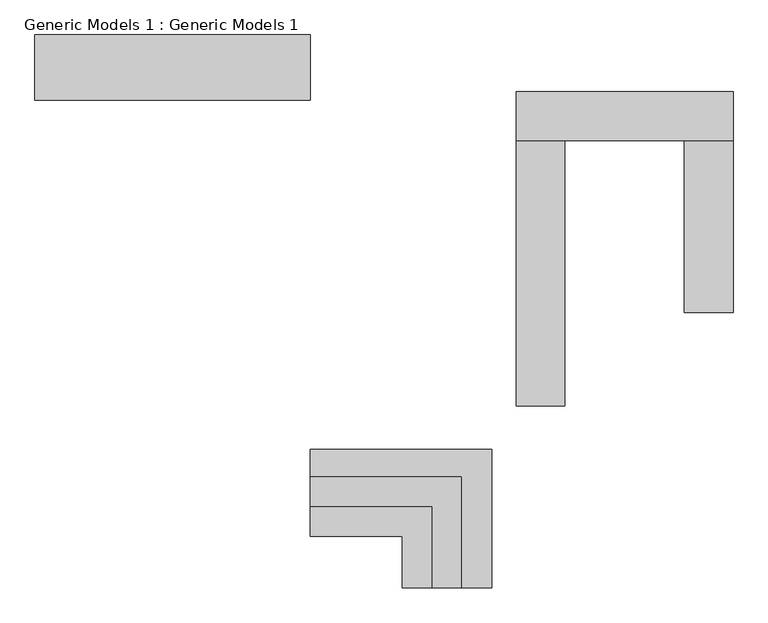
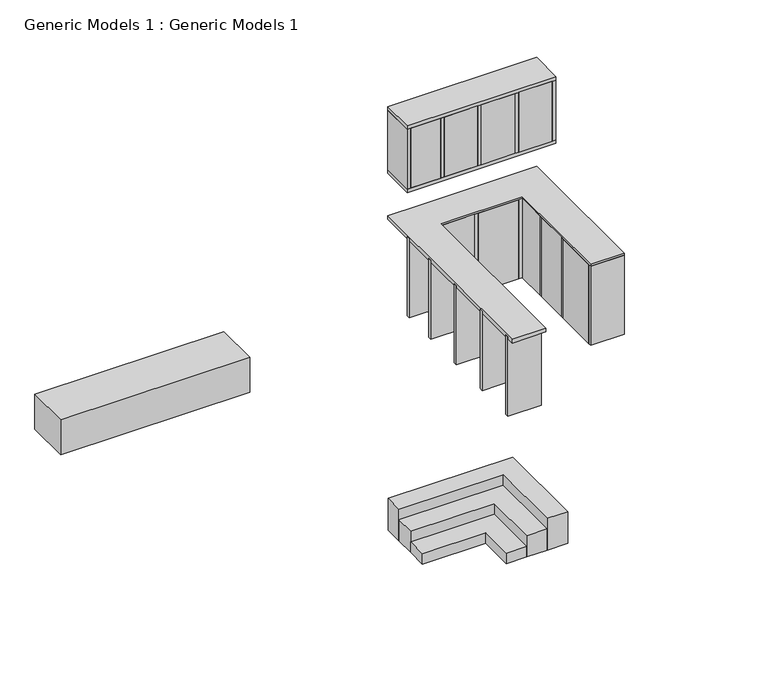
"""IFC4 building model written with IfcOpenShell, lengths in millimetres: proxy geometry, Generic Models 1 : Generic Models 1."""

from ifc_helpers import new_model, si_unit, frame, origin, place, context, project, spatial, polyline, outline, extrude, source, transform, mapped, element, save


def generic_models_1_generic_models_1_30c65cec(model_context):
    return source(origin(), model_context, "Body", "SweptSolid", [
        extrude(outline(polyline([(-6395.1591227, 5407.3642852), (-6395.1591227, 4797.7642852), (-8973.2591227, 4797.7642852), (-8973.2591227, 5407.3642852), (-6395.1591227, 5407.3642852)])), frame((0.0, 0.0, -609.6), z_axis=(0.0, 0.0, 1.0), x_axis=(1.0, 0.0, 0.0)), (0.0, 0.0, 1.0), 508.0),
        extrude(outline(polyline([(-5252.1591227, 987.7642852), (-5252.1591227, 225.7642852), (-5531.5591227, 225.7642852), (-5531.5591227, 708.3642852), (-6395.1591227, 708.3642852), (-6395.1591227, 987.7642852), (-5252.1591227, 987.7642852)])), frame((0.0, 0.0, -609.6), z_axis=(0.0, 0.0, 1.0), x_axis=(1.0, 0.0, 0.0)), (0.0, 0.0, 1.0), 152.4),
        extrude(outline(polyline([(-6395.1591227, 987.7642852), (-6395.1591227, 1267.1642852), (-4972.7591227, 1267.1642852), (-4972.7591227, 225.7642852), (-5252.1591227, 225.7642852), (-5252.1591227, 987.7642852), (-6395.1591227, 987.7642852)])), frame((0.0, 0.0, -609.6), z_axis=(0.0, 0.0, 1.0), x_axis=(1.0, 0.0, 0.0)), (0.0, 0.0, 1.0), 304.8),
        extrude(outline(polyline([(-4693.3591227, 1521.1642852), (-4693.3591227, 225.7642852), (-4972.7591227, 225.7642852), (-4972.7591227, 1267.1642852), (-6395.1591227, 1267.1642852), (-6395.1591227, 1521.1642852), (-4693.3591227, 1521.1642852)])), frame((0.0, 0.0, -609.6), z_axis=(0.0, 0.0, 1.0), x_axis=(1.0, 0.0, 0.0)), (0.0, 0.0, 1.0), 457.2),
        extrude(outline(polyline([(-4007.5591227, 4416.7642852), (-4413.9591227, 4416.7642852), (-4413.9591227, 4436.1688715), (-4007.5591227, 4436.1688715), (-4007.5591227, 4416.7642852)])), frame((0.0, 0.0, 1879.6), z_axis=(0.0, 0.0, 1.0), x_axis=(1.0, 0.0, 0.0)), (0.0, 0.0, 1.0), 863.6),
        extrude(outline(polyline([(-3499.5591227, 4416.7642852), (-3956.7591227, 4416.7642852), (-3956.7591227, 4436.1688715), (-3499.5591227, 4436.1688715), (-3499.5591227, 4416.7642852)])), frame((0.0, 0.0, 1879.6), z_axis=(0.0, 0.0, 1.0), x_axis=(1.0, 0.0, 0.0)), (0.0, 0.0, 1.0), 863.6),
        extrude(outline(polyline([(-2991.5591227, 4416.7642852), (-3448.7591227, 4416.7642852), (-3448.7591227, 4436.1688715), (-2991.5591227, 4436.1688715), (-2991.5591227, 4416.7642852)])), frame((0.0, 0.0, 1879.6), z_axis=(0.0, 0.0, 1.0), x_axis=(1.0, 0.0, 0.0)), (0.0, 0.0, 1.0), 863.6),
        extrude(outline(polyline([(-2483.5591227, 4416.7642852), (-2940.7591227, 4416.7642852), (-2940.7591227, 4436.1688715), (-2483.5591227, 4436.1688715), (-2483.5591227, 4416.7642852)])), frame((0.0, 0.0, 1879.6), z_axis=(0.0, 0.0, 1.0), x_axis=(1.0, 0.0, 0.0)), (0.0, 0.0, 1.0), 863.6),
        extrude(outline(polyline([(-2432.7591227, 4873.9642852), (-2432.7591227, 4416.7642852), (-4464.7591227, 4416.7642852), (-4464.7591227, 4873.9642852), (-2432.7591227, 4873.9642852)])), frame((0.0, 0.0, 2743.2), z_axis=(0.0, 0.0, 1.0), x_axis=(1.0, 0.0, 0.0)), (0.0, 0.0, 1.0), 50.8),
        extrude(outline(polyline([(-4413.9591227, 4873.9642852), (-4413.9591227, 4416.7642852), (-4464.7591227, 4416.7642852), (-4464.7591227, 4873.9642852), (-4413.9591227, 4873.9642852)])), frame((0.0, 0.0, 1879.6), z_axis=(0.0, 0.0, 1.0), x_axis=(1.0, 0.0, 0.0)), (0.0, 0.0, 1.0), 863.6),
        extrude(outline(polyline([(-3956.7591227, 4873.9642852), (-3956.7591227, 4416.7642852), (-4007.5591227, 4416.7642852), (-4007.5591227, 4873.9642852), (-3956.7591227, 4873.9642852)])), frame((0.0, 0.0, 1879.6), z_axis=(0.0, 0.0, 1.0), x_axis=(1.0, 0.0, 0.0)), (0.0, 0.0, 1.0), 863.6),
        extrude(outline(polyline([(-3448.7591227, 4873.9642852), (-3448.7591227, 4416.7642852), (-3499.5591227, 4416.7642852), (-3499.5591227, 4873.9642852), (-3448.7591227, 4873.9642852)])), frame((0.0, 0.0, 1879.6), z_axis=(0.0, 0.0, 1.0), x_axis=(1.0, 0.0, 0.0)), (0.0, 0.0, 1.0), 863.6),
        extrude(outline(polyline([(-2991.5591227, 4873.9642852), (-2940.7591227, 4873.9642852), (-2940.7591227, 4416.7642852), (-2991.5591227, 4416.7642852), (-2991.5591227, 4873.9642852)])), frame((0.0, 0.0, 1879.6), z_axis=(0.0, 0.0, 1.0), x_axis=(1.0, 0.0, 0.0)), (0.0, 0.0, 1.0), 863.6),
        extrude(outline(polyline([(-2483.5591227, 4873.9642852), (-2432.7591227, 4873.9642852), (-2432.7591227, 4416.7642852), (-2483.5591227, 4416.7642852), (-2483.5591227, 4873.9642852)])), frame((0.0, 0.0, 1879.6), z_axis=(0.0, 0.0, 1.0), x_axis=(1.0, 0.0, 0.0)), (0.0, 0.0, 1.0), 863.6),
        extrude(outline(polyline([(-2432.7591227, 4873.9642852), (-2432.7591227, 4416.7642852), (-4464.7591227, 4416.7642852), (-4464.7591227, 4873.9642852), (-2432.7591227, 4873.9642852)])), frame((0.0, 0.0, 1828.8), z_axis=(0.0, 0.0, 1.0), x_axis=(1.0, 0.0, 0.0)), (0.0, 0.0, 1.0), 50.8),
        extrude(outline(polyline([(-4058.3591227, 2079.9642852), (-4058.3591227, 2638.7642852), (-4007.5591227, 2638.7642852), (-4007.5591227, 2079.9642852), (-4058.3591227, 2079.9642852)])), frame((0.0, 0.0, 50.8), z_axis=(0.0, 0.0, 1.0), x_axis=(1.0, 0.0, 0.0)), (0.0, 0.0, 1.0), 1143.0),
        extrude(outline(polyline([(-4058.3591227, 2689.5642852), (-4058.3591227, 3248.3642852), (-4007.5591227, 3248.3642852), (-4007.5591227, 2689.5642852), (-4058.3591227, 2689.5642852)])), frame((0.0, 0.0, 50.8), z_axis=(0.0, 0.0, 1.0), x_axis=(1.0, 0.0, 0.0)), (0.0, 0.0, 1.0), 1143.0),
        extrude(outline(polyline([(-4058.3591227, 3299.1642852), (-4058.3591227, 3857.9642852), (-4007.5591227, 3857.9642852), (-4007.5591227, 3299.1642852), (-4058.3591227, 3299.1642852)])), frame((0.0, 0.0, 50.8), z_axis=(0.0, 0.0, 1.0), x_axis=(1.0, 0.0, 0.0)), (0.0, 0.0, 1.0), 1143.0),
        extrude(outline(polyline([(-4058.3591227, 3908.7642852), (-4058.3591227, 4365.9642852), (-4007.5591227, 4365.9642852), (-4007.5591227, 3908.7642852), (-4058.3591227, 3908.7642852)])), frame((0.0, 0.0, 50.8), z_axis=(0.0, 0.0, 1.0), x_axis=(1.0, 0.0, 0.0)), (0.0, 0.0, 1.0), 1143.0),
        extrude(outline(polyline([(-4007.5591227, 4416.7642852), (-4007.5591227, 4455.5734579), (-3544.3461758, 4455.5734579), (-3544.3461758, 4416.7642852), (-4007.5591227, 4416.7642852)])), frame((0.0, 0.0, 50.8), z_axis=(0.0, 0.0, 1.0), x_axis=(1.0, 0.0, 0.0)), (0.0, 0.0, 1.0), 1143.0),
        extrude(outline(polyline([(-3493.5461758, 4416.7642852), (-3493.5461758, 4455.5734579), (-2940.7591227, 4455.5734579), (-2940.7591227, 4416.7642852), (-3493.5461758, 4416.7642852)])), frame((0.0, 0.0, 50.8), z_axis=(0.0, 0.0, 1.0), x_axis=(1.0, 0.0, 0.0)), (0.0, 0.0, 1.0), 1143.0),
        extrude(outline(polyline([(-2865.8793637, 4010.3642852), (-2889.9591227, 4010.3642852), (-2889.9591227, 4416.7642852), (-2865.8793637, 4416.7642852), (-2865.8793637, 4010.3642852)])), frame((0.0, 0.0, 50.8), z_axis=(0.0, 0.0, 1.0), x_axis=(1.0, 0.0, 0.0)), (0.0, 0.0, 1.0), 1143.0),
        extrude(outline(polyline([(-2865.8793637, 3502.3642852), (-2889.9591227, 3502.3642852), (-2889.9591227, 3959.5642852), (-2865.8793637, 3959.5642852), (-2865.8793637, 3502.3642852)])), frame((0.0, 0.0, 50.8), z_axis=(0.0, 0.0, 1.0), x_axis=(1.0, 0.0, 0.0)), (0.0, 0.0, 1.0), 1143.0),
        extrude(outline(polyline([(-2865.8793637, 2841.9642852), (-2889.9591227, 2841.9642852), (-2889.9591227, 3451.5642852), (-2865.8793637, 3451.5642852), (-2865.8793637, 2841.9642852)])), frame((0.0, 0.0, 50.8), z_axis=(0.0, 0.0, 1.0), x_axis=(1.0, 0.0, 0.0)), (0.0, 0.0, 1.0), 1143.0),
        extrude(outline(polyline([(-4007.5591227, 2029.1642852), (-4464.7591227, 2029.1642852), (-4464.7591227, 2079.9642852), (-4007.5591227, 2079.9642852), (-4007.5591227, 2029.1642852)])), frame((0.0, 0.0, 50.8), z_axis=(0.0, 0.0, 1.0), x_axis=(1.0, 0.0, 0.0)), (0.0, 0.0, 1.0), 1143.0),
        extrude(outline(polyline([(-4007.5591227, 2638.7642852), (-4464.7591227, 2638.7642852), (-4464.7591227, 2689.5642852), (-4007.5591227, 2689.5642852), (-4007.5591227, 2638.7642852)])), frame((0.0, 0.0, 50.8), z_axis=(0.0, 0.0, 1.0), x_axis=(1.0, 0.0, 0.0)), (0.0, 0.0, 1.0), 1143.0),
        extrude(outline(polyline([(-4007.5591227, 3248.3642852), (-4464.7591227, 3248.3642852), (-4464.7591227, 3299.1642852), (-4007.5591227, 3299.1642852), (-4007.5591227, 3248.3642852)])), frame((0.0, 0.0, 50.8), z_axis=(0.0, 0.0, 1.0), x_axis=(1.0, 0.0, 0.0)), (0.0, 0.0, 1.0), 1143.0),
        extrude(outline(polyline([(-4007.5591227, 3857.9642852), (-4464.7591227, 3857.9642852), (-4464.7591227, 3908.7642852), (-4007.5591227, 3908.7642852), (-4007.5591227, 3857.9642852)])), frame((0.0, 0.0, 50.8), z_axis=(0.0, 0.0, 1.0), x_axis=(1.0, 0.0, 0.0)), (0.0, 0.0, 1.0), 1143.0),
        extrude(outline(polyline([(-4007.5591227, 4365.9642852), (-4464.7591227, 4365.9642852), (-4464.7591227, 4416.7642852), (-4007.5591227, 4416.7642852), (-4007.5591227, 4365.9642852)])), frame((0.0, 0.0, 50.8), z_axis=(0.0, 0.0, 1.0), x_axis=(1.0, 0.0, 0.0)), (0.0, 0.0, 1.0), 1143.0),
        extrude(outline(polyline([(-3544.3461758, 4416.7642852), (-3544.3461758, 4873.9642852), (-3493.5461758, 4873.9642852), (-3493.5461758, 4416.7642852), (-3544.3461758, 4416.7642852)])), frame((0.0, 0.0, 50.8), z_axis=(0.0, 0.0, 1.0), x_axis=(1.0, 0.0, 0.0)), (0.0, 0.0, 1.0), 1143.0),
        extrude(outline(polyline([(-2940.7591227, 4416.7642852), (-2940.7591227, 4873.9642852), (-2889.9591227, 4873.9642852), (-2889.9591227, 4416.7642852), (-2940.7591227, 4416.7642852)])), frame((0.0, 0.0, 50.8), z_axis=(0.0, 0.0, 1.0), x_axis=(1.0, 0.0, 0.0)), (0.0, 0.0, 1.0), 1143.0),
        extrude(outline(polyline([(-2432.7591227, 2803.8642852), (-2889.9591227, 2803.8642852), (-2889.9591227, 2841.9642852), (-2432.7591227, 2841.9642852), (-2432.7591227, 2803.8642852)])), frame((0.0, 0.0, 50.8), z_axis=(0.0, 0.0, 1.0), x_axis=(1.0, 0.0, 0.0)), (0.0, 0.0, 1.0), 1143.0),
        extrude(outline(polyline([(-2432.7591227, 3451.5642852), (-2889.9591227, 3451.5642852), (-2889.9591227, 3502.3642852), (-2432.7591227, 3502.3642852), (-2432.7591227, 3451.5642852)])), frame((0.0, 0.0, 50.8), z_axis=(0.0, 0.0, 1.0), x_axis=(1.0, 0.0, 0.0)), (0.0, 0.0, 1.0), 1143.0),
        extrude(outline(polyline([(-2432.7591227, 3959.5642852), (-2889.9591227, 3959.5642852), (-2889.9591227, 4010.3642852), (-2432.7591227, 4010.3642852), (-2432.7591227, 3959.5642852)])), frame((0.0, 0.0, 50.8), z_axis=(0.0, 0.0, 1.0), x_axis=(1.0, 0.0, 0.0)), (0.0, 0.0, 1.0), 1143.0),
        extrude(outline(polyline([(-4007.5591227, 1927.5642852), (-4464.7591227, 1927.5642852), (-4464.7591227, 4873.9642852), (-4008.5861775, 4873.9642852), (-2432.7591227, 4873.9642852), (-2432.7591227, 4519.1838129), (-2432.7591227, 2803.8642852), (-2889.9591227, 2803.8642852), (-2889.9591227, 4416.7642852), (-4007.5591227, 4416.7642852), (-4007.5591227, 1927.5642852)])), frame((0.0, 0.0, 1168.4), z_axis=(0.0, 0.0, 1.0), x_axis=(1.0, 0.0, 0.0)), (0.0, 0.0, 1.0), 50.8),
    ])


if __name__ == "__main__":
    model = new_model("IFC4")
    model_context = context("Model", 3, world=origin())
    ifc_project = project(units=[si_unit("LENGTHUNIT", "METRE", prefix="MILLI")], contexts=[model_context])
    site = spatial("IfcSite", under=ifc_project)
    building = spatial("IfcBuilding", under=site)
    placement = place(None, origin())
    generic_models_1_generic_models_1_shape = generic_models_1_generic_models_1_30c65cec(model_context)
    element("IfcBuildingElementProxy", 1, Name="Generic Models 1 : Generic Models 1", ObjectType="Generic Models 1 : Generic Models 1", at=placement, inside=building, context=model_context, shape_type="MappedRepresentation", body=[
        mapped(generic_models_1_generic_models_1_shape, transform((0.0, 0.0, 0.0), x_axis=(1.0, 0.0, 0.0), y_axis=(0.0, 1.0, 0.0), z_axis=(0.0, 0.0, 1.0))),
    ])
    save(model, "model.ifc")

# Revit data of these elements
# Element 1 (IfcBuildingElementProxy, "Generic Models 1 : Generic Models 1")
#   Materials on its faces: "Grass"
# Materials
#   "Grass": class "Generic", colour RGB 27 35 14, transparency 0, Description = "Physical material.", Cost = 0
